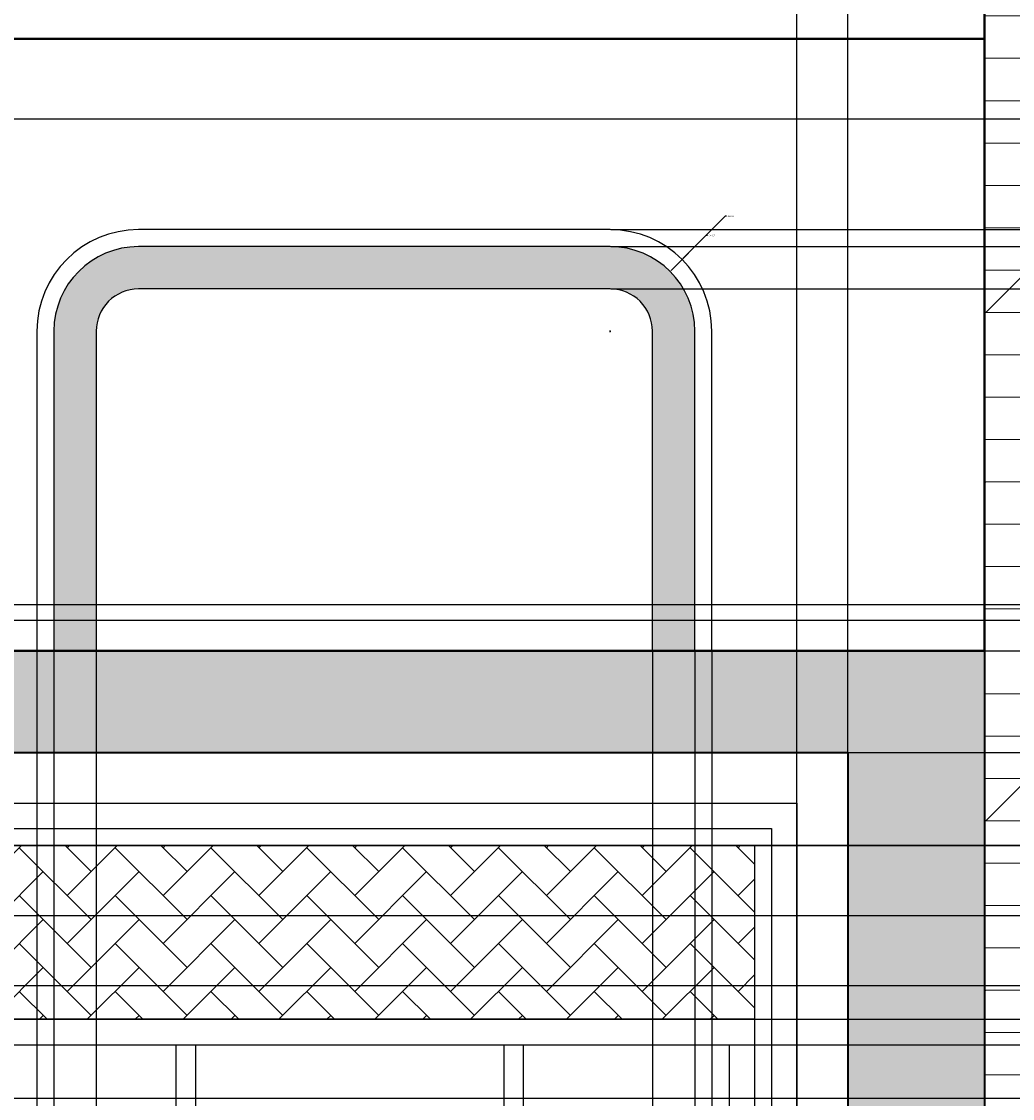
# Model space of a CAD drawing. Units: inches. Extents: x -13 to 630, y -103 to 275.
# Tile 4 of 9: x 51 to 168, y 72 to 199. Entities that reach past the tile are written whole.
import ezdxf

# ---------------------------------------------------------------- set-up
doc = ezdxf.new("R2010")
doc.units = ezdxf.units.IN
doc.header["$MEASUREMENT"] = 0
for name, color, linetype, lineweight in [('A-ANNO-DIMS', 2, 'Continuous', 18), ('A-ELEV', 7, 'Continuous', 35), ('A-ELEV-PATT', 8, 'Continuous', 13), ('A-GLAZ', 4, 'Continuous', 25)]:
    doc.layers.add(name, color=color, linetype=linetype, lineweight=lineweight)
doc.styles.get("Standard").update_dxf_attribs({"font": 'arial.ttf'})
doc.dimstyles.get("Standard").update_dxf_attribs({"dimtxt": 0.18, "dimasz": 0.18, "dimexe": 0.18, "dimexo": 0.0625, "dimgap": 0.09, "dimtad": 0, "dimtih": 1, "dimtoh": 1, "dimdec": 4, "dimzin": 0, "dimdsep": 46, "dimtxsty": 'Standard', "dimcen": 0.09, "dimadec": 0, "dimazin": 0, "dimtfac": 1, "dimtdec": 4, "dimtofl": 0, "dimtmove": 0, "dimatfit": 3, "dimfxl": 1, "dimtolj": 1, "dimtzin": 0, "dimarcsym": 0})

# ---------------------------------------------------------------- blocks, each defined once
blk = doc.blocks.new('WIN-GROUND')
for points in [[(0, 0), (0, 102), (108, 102), (108, 0)], [(3, 0), (3, 99), (105, 99), (105, 0)], [(5, 0), (5, 97), (103, 97), (103, 0)], [(34.74, 56.82), (34.74, 73.49), (37, 73.49), (37, 56.82)], [(73.43, 56.82), (73.43, 73.49), (75.7, 73.49), (75.7, 56.82)], [(34.74, 55.51), (8, 55.51), (8, 56.82), (34.74, 56.82)], [(37, 56.82), (73.43, 56.82)], [(75.7, 56.82), (100, 56.82), (100, 55.51), (75.7, 55.51)], [(34.74, 21.58), (34.74, 55.51)], [(37, 55.51), (37, 21.58)], [(73.43, 55.51), (37, 55.51)], [(73.43, 21.58), (73.43, 55.51)], [(75.7, 55.51), (75.7, 21.58)], [(34.74, 20.27), (8, 20.27), (8, 21.58), (34.74, 21.58)], [(37, 21.58), (73.43, 21.58)], [(75.7, 21.58), (100, 21.58), (100, 20.27), (75.7, 20.27)], [(37, 20.27), (37, 3), (34.74, 3), (34.74, 20.27)], [(73.43, 20.27), (37, 20.27)], [(75.7, 20.27), (75.7, 3), (73.43, 3), (73.43, 20.27)]]:
    blk.add_lwpolyline(points)
for points in [[(5, 97), (103, 97), (103, 76.49), (5, 76.49)], [(5, 76.49), (103, 76.49), (103, 0), (5, 0)], [(8, 73.49), (100, 73.49), (100, 3), (8, 3)]]:
    blk.add_lwpolyline(points, close=True)
blk = doc.blocks.new('*D8')
at = {"layer": 'A-ANNO-DIMS', "color": 0, "lineweight": -2, "transparency": 16777216}
for p, q in [((142.71, 5.14), (142.71, 275.01)), ((142.89, 274.83), (153.31, 274.83)), ((164.66, 274.83), (154.24, 274.83)), ((164.84, 5.14), (164.84, 275.01))]:
    blk.add_line(p, q, dxfattribs=at)
at = {"layer": 'A-ANNO-DIMS', "color": 0, "transparency": 16777216}
for points in [[(142.89, 274.86), (142.89, 274.8), (142.71, 274.83)], [(164.66, 274.86), (164.66, 274.8), (164.84, 274.83)]]:
    blk.add_solid(points, dxfattribs=at)
at = {"layer": 'Defpoints', "color": 0, "transparency": 16777216}
for p in [(164.84, 274.83), (142.71, 5.08), (164.84, 5.08)]:
    blk.add_point(p, dxfattribs=at)
at = {"layer": 'A-ANNO-DIMS', "color": 0, "transparency": 16777216, "insert": (153.78, 274.83), "char_height": 0.18, "attachment_point": 5}
blk.add_mtext('\\A1;22.133', dxfattribs=at)
blk = doc.blocks.new('*D41')
at = {"layer": 'A-ANNO-DIMS', "color": 0, "lineweight": -2, "transparency": 16777216}
for p, q in [((205.96, 72.22), (-13.22, 72.22)), ((-13.04, 72.04), (-13.04, 71.07)), ((-13.04, 69.73), (-13.04, 70.7)), ((205.96, 69.55), (-13.22, 69.55))]:
    blk.add_line(p, q, dxfattribs=at)
at = {"layer": 'A-ANNO-DIMS', "color": 0, "transparency": 16777216}
for points in [[(-13.07, 72.04), (-13.01, 72.04), (-13.04, 72.22)], [(-13.07, 69.73), (-13.01, 69.73), (-13.04, 69.55)]]:
    blk.add_solid(points, dxfattribs=at)
at = {"layer": 'Defpoints', "color": 0, "transparency": 16777216}
for p in [(-13.04, 72.22), (206.02, 72.22), (206.02, 69.55)]:
    blk.add_point(p, dxfattribs=at)
at = {"layer": 'A-ANNO-DIMS', "color": 0, "transparency": 16777216, "insert": (-13.04, 70.88), "char_height": 0.18, "attachment_point": 5}
blk.add_mtext('\\A1;2.68', dxfattribs=at)
blk = doc.blocks.new('*D42')
at = {"layer": 'A-ANNO-DIMS', "color": 0, "lineweight": -2, "transparency": 16777216}
for p, q in [((205.96, 85.52), (-13.22, 85.52)), ((-13.04, 85.34), (-13.04, 79.05)), ((-13.04, 72.4), (-13.04, 78.69)), ((205.96, 72.22), (-13.22, 72.22))]:
    blk.add_line(p, q, dxfattribs=at)
at = {"layer": 'A-ANNO-DIMS', "color": 0, "transparency": 16777216}
for points in [[(-13.07, 85.34), (-13.01, 85.34), (-13.04, 85.52)], [(-13.07, 72.4), (-13.01, 72.4), (-13.04, 72.22)]]:
    blk.add_solid(points, dxfattribs=at)
at = {"layer": 'Defpoints', "color": 0, "transparency": 16777216}
for p in [(-13.04, 85.52), (206.02, 85.52), (206.02, 72.22)]:
    blk.add_point(p, dxfattribs=at)
at = {"layer": 'A-ANNO-DIMS', "color": 0, "transparency": 16777216, "insert": (-13.04, 78.87), "char_height": 0.18, "attachment_point": 5}
blk.add_mtext('\\A1;13.297', dxfattribs=at)
blk = doc.blocks.new('*D43')
at = {"layer": 'A-ANNO-DIMS', "color": 0, "lineweight": -2, "transparency": 16777216}
for p, q in [((205.96, 93.8), (-13.22, 93.8)), ((-13.04, 93.62), (-13.04, 89.84)), ((-13.04, 85.7), (-13.04, 89.48)), ((205.96, 85.52), (-13.22, 85.52))]:
    blk.add_line(p, q, dxfattribs=at)
at = {"layer": 'A-ANNO-DIMS', "color": 0, "transparency": 16777216}
for points in [[(-13.07, 93.62), (-13.01, 93.62), (-13.04, 93.8)], [(-13.07, 85.7), (-13.01, 85.7), (-13.04, 85.52)]]:
    blk.add_solid(points, dxfattribs=at)
at = {"layer": 'Defpoints', "color": 0, "transparency": 16777216}
for p in [(-13.04, 93.8), (206.02, 93.8), (206.02, 85.52)]:
    blk.add_point(p, dxfattribs=at)
at = {"layer": 'A-ANNO-DIMS', "color": 0, "transparency": 16777216, "insert": (-13.04, 89.66), "char_height": 0.18, "attachment_point": 5}
blk.add_mtext('\\A1;8.28', dxfattribs=at)
blk = doc.blocks.new('*D44')
at = {"layer": 'A-ANNO-DIMS', "color": 0, "lineweight": -2, "transparency": 16777216}
for p, q in [((205.96, 102.08), (-13.22, 102.08)), ((-13.04, 101.9), (-13.04, 98.12)), ((-13.04, 93.98), (-13.04, 97.76)), ((205.96, 93.8), (-13.22, 93.8))]:
    blk.add_line(p, q, dxfattribs=at)
at = {"layer": 'A-ANNO-DIMS', "color": 0, "transparency": 16777216}
for points in [[(-13.07, 101.9), (-13.01, 101.9), (-13.04, 102.08)], [(-13.07, 93.98), (-13.01, 93.98), (-13.04, 93.8)]]:
    blk.add_solid(points, dxfattribs=at)
at = {"layer": 'Defpoints', "color": 0, "transparency": 16777216}
for p in [(-13.04, 102.08), (206.02, 102.08), (206.02, 93.8)]:
    blk.add_point(p, dxfattribs=at)
at = {"layer": 'A-ANNO-DIMS', "color": 0, "transparency": 16777216, "insert": (-13.04, 97.94), "char_height": 0.18, "attachment_point": 5}
blk.add_mtext('\\A1;8.28', dxfattribs=at)
blk = doc.blocks.new('*D45')
at = {"layer": 'A-ANNO-DIMS', "color": 0, "lineweight": -2, "transparency": 16777216}
for p, q in [((205.96, 128.66), (-13.22, 128.66)), ((-13.04, 128.48), (-13.04, 115.55)), ((-13.04, 102.26), (-13.04, 115.19)), ((205.96, 102.08), (-13.22, 102.08))]:
    blk.add_line(p, q, dxfattribs=at)
at = {"layer": 'A-ANNO-DIMS', "color": 0, "transparency": 16777216}
for points in [[(-13.07, 128.48), (-13.01, 128.48), (-13.04, 128.66)], [(-13.07, 102.26), (-13.01, 102.26), (-13.04, 102.08)]]:
    blk.add_solid(points, dxfattribs=at)
at = {"layer": 'Defpoints', "color": 0, "transparency": 16777216}
for p in [(-13.04, 128.66), (206.02, 128.66), (206.02, 102.08)]:
    blk.add_point(p, dxfattribs=at)
at = {"layer": 'A-ANNO-DIMS', "color": 0, "transparency": 16777216, "insert": (-13.04, 115.37), "char_height": 0.18, "attachment_point": 5}
blk.add_mtext('\\A1;26.574', dxfattribs=at)
blk = doc.blocks.new('*D46')
at = {"layer": 'A-ANNO-DIMS', "color": 0, "lineweight": -2, "transparency": 16777216}
for p, q in [((205.96, 130.51), (-13.22, 130.51)), ((-13.04, 130.33), (-13.04, 129.76)), ((205.96, 128.66), (-13.22, 128.66)), ((-13.04, 128.84), (-13.04, 129.4))]:
    blk.add_line(p, q, dxfattribs=at)
at = {"layer": 'A-ANNO-DIMS', "color": 0, "transparency": 16777216}
for points in [[(-13.07, 130.33), (-13.01, 130.33), (-13.04, 130.51)], [(-13.07, 128.84), (-13.01, 128.84), (-13.04, 128.66)]]:
    blk.add_solid(points, dxfattribs=at)
at = {"layer": 'Defpoints', "color": 0, "transparency": 16777216}
for p in [(-13.04, 130.51), (206.02, 130.51), (206.02, 128.66)]:
    blk.add_point(p, dxfattribs=at)
at = {"layer": 'A-ANNO-DIMS', "color": 0, "transparency": 16777216, "insert": (-13.04, 129.58), "char_height": 0.18, "attachment_point": 5}
blk.add_mtext('\\A1;1.854', dxfattribs=at)
blk = doc.blocks.new('*D47')
at = {"layer": 'A-ANNO-DIMS', "color": 0, "lineweight": -2, "transparency": 16777216}
for p, q in [((252.21, 187.83), (-13.22, 187.83)), ((-13.04, 187.65), (-13.04, 159.35)), ((-13.04, 130.69), (-13.04, 158.99)), ((205.96, 130.51), (-13.22, 130.51))]:
    blk.add_line(p, q, dxfattribs=at)
at = {"layer": 'A-ANNO-DIMS', "color": 0, "transparency": 16777216}
for points in [[(-13.07, 187.65), (-13.01, 187.65), (-13.04, 187.83)], [(-13.07, 130.69), (-13.01, 130.69), (-13.04, 130.51)]]:
    blk.add_solid(points, dxfattribs=at)
at = {"layer": 'Defpoints', "color": 0, "transparency": 16777216}
for p in [(-13.04, 187.83), (252.27, 187.83), (206.02, 130.51)]:
    blk.add_point(p, dxfattribs=at)
at = {"layer": 'A-ANNO-DIMS', "color": 0, "transparency": 16777216, "insert": (-13.04, 159.17), "char_height": 0.18, "attachment_point": 5}
blk.add_mtext('\\A1;57.32', dxfattribs=at)
blk = doc.blocks.new('*D70')
at = {"layer": 'A-ANNO-DIMS', "color": 0, "lineweight": -2, "transparency": 16777216}
for p, q in [((142.71, 107.14), (142.71, 275.01)), ((142.89, 274.83), (145.56, 274.83)), ((148.53, 274.83), (145.86, 274.83)), ((148.71, 113.14), (148.71, 275.01))]:
    blk.add_line(p, q, dxfattribs=at)
at = {"layer": 'A-ANNO-DIMS', "color": 0, "transparency": 16777216}
for points in [[(142.89, 274.86), (142.89, 274.8), (142.71, 274.83)], [(148.53, 274.86), (148.53, 274.8), (148.71, 274.83)]]:
    blk.add_solid(points, dxfattribs=at)
at = {"layer": 'Defpoints', "color": 0, "transparency": 16777216}
for p in [(148.71, 274.83), (148.71, 113.08), (142.71, 107.08)]:
    blk.add_point(p, dxfattribs=at)
at = {"layer": 'A-ANNO-DIMS', "color": 0, "transparency": 16777216, "insert": (145.71, 274.83), "char_height": 0.18, "attachment_point": 5}
blk.add_mtext('\\A1;6', dxfattribs=at)
blk = doc.blocks.new('*D83')
at = {"layer": 'A-ANNO-DIMS', "color": 0, "lineweight": -2, "transparency": 16777216}
for p, q in [((134.77, 78.57), (630.03, 78.57)), ((629.85, 78.39), (629.85, 70.42)), ((629.85, 62.08), (629.85, 70.05)), ((134.77, 61.9), (630.03, 61.9))]:
    blk.add_line(p, q, dxfattribs=at)
at = {"layer": 'A-ANNO-DIMS', "color": 0, "transparency": 16777216}
for points in [[(629.82, 78.39), (629.88, 78.39), (629.85, 78.57)], [(629.82, 62.08), (629.88, 62.08), (629.85, 61.9)]]:
    blk.add_solid(points, dxfattribs=at)
at = {"layer": 'Defpoints', "color": 0, "transparency": 16777216}
for p in [(134.71, 78.57), (629.85, 78.57), (134.71, 61.9)]:
    blk.add_point(p, dxfattribs=at)
at = {"layer": 'A-ANNO-DIMS', "color": 0, "transparency": 16777216, "insert": (629.85, 70.24), "char_height": 0.18, "attachment_point": 5}
blk.add_mtext('\\A1;16.67', dxfattribs=at)
blk = doc.blocks.new('*D84')
at = {"layer": 'A-ANNO-DIMS', "color": 0, "lineweight": -2, "transparency": 16777216}
for p, q in [((137.77, 81.57), (630.03, 81.57)), ((629.85, 81.39), (629.85, 80.25)), ((629.85, 78.75), (629.85, 79.89)), ((134.77, 78.57), (630.03, 78.57))]:
    blk.add_line(p, q, dxfattribs=at)
at = {"layer": 'A-ANNO-DIMS', "color": 0, "transparency": 16777216}
for points in [[(629.82, 81.39), (629.88, 81.39), (629.85, 81.57)], [(629.82, 78.75), (629.88, 78.75), (629.85, 78.57)]]:
    blk.add_solid(points, dxfattribs=at)
at = {"layer": 'Defpoints', "color": 0, "transparency": 16777216}
for p in [(137.71, 81.57), (629.85, 81.57), (134.71, 78.57)]:
    blk.add_point(p, dxfattribs=at)
at = {"layer": 'A-ANNO-DIMS', "color": 0, "transparency": 16777216, "insert": (629.85, 80.07), "char_height": 0.18, "attachment_point": 5}
blk.add_mtext('\\A1;3', dxfattribs=at)
blk = doc.blocks.new('*D85')
at = {"layer": 'A-ANNO-DIMS', "color": 0, "lineweight": -2, "transparency": 16777216}
for p, q in [((137.77, 102.08), (630.03, 102.08)), ((629.85, 101.9), (629.85, 92.01)), ((629.85, 81.75), (629.85, 91.64)), ((137.77, 81.57), (630.03, 81.57))]:
    blk.add_line(p, q, dxfattribs=at)
at = {"layer": 'A-ANNO-DIMS', "color": 0, "transparency": 16777216}
for points in [[(629.82, 101.9), (629.88, 101.9), (629.85, 102.08)], [(629.82, 81.75), (629.88, 81.75), (629.85, 81.57)]]:
    blk.add_solid(points, dxfattribs=at)
at = {"layer": 'Defpoints', "color": 0, "transparency": 16777216}
for p in [(137.71, 102.08), (629.85, 102.08), (137.71, 81.57)]:
    blk.add_point(p, dxfattribs=at)
at = {"layer": 'A-ANNO-DIMS', "color": 0, "transparency": 16777216, "insert": (629.85, 91.83), "char_height": 0.18, "attachment_point": 5}
blk.add_mtext('\\A1;20.51', dxfattribs=at)
blk = doc.blocks.new('*D86')
at = {"layer": 'A-ANNO-DIMS', "color": 0, "lineweight": -2, "transparency": 16777216}
for p, q in [((148.77, 113.08), (630.03, 113.08)), ((629.85, 112.9), (629.85, 107.76)), ((629.85, 102.26), (629.85, 107.4)), ((137.77, 102.08), (630.03, 102.08))]:
    blk.add_line(p, q, dxfattribs=at)
at = {"layer": 'A-ANNO-DIMS', "color": 0, "transparency": 16777216}
for points in [[(629.82, 112.9), (629.88, 112.9), (629.85, 113.08)], [(629.82, 102.26), (629.88, 102.26), (629.85, 102.08)]]:
    blk.add_solid(points, dxfattribs=at)
at = {"layer": 'Defpoints', "color": 0, "transparency": 16777216}
for p in [(148.71, 113.08), (629.85, 113.08), (137.71, 102.08)]:
    blk.add_point(p, dxfattribs=at)
at = {"layer": 'A-ANNO-DIMS', "color": 0, "transparency": 16777216, "insert": (629.85, 107.58), "char_height": 0.18, "attachment_point": 5}
blk.add_mtext('\\A1;11', dxfattribs=at)
blk = doc.blocks.new('*D106')
at = {"layer": 'A-ANNO-DIMS', "color": 0, "lineweight": -2, "transparency": 16777216}
for p, q in [((42.29, 125.02), (42.29, -103.45)), ((53, 125.02), (53, -103.45)), ((42.47, -103.27), (47.27, -103.27)), ((52.82, -103.27), (48.01, -103.27))]:
    blk.add_line(p, q, dxfattribs=at)
at = {"layer": 'A-ANNO-DIMS', "color": 0, "transparency": 16777216}
for points in [[(42.47, -103.24), (42.47, -103.3), (42.29, -103.27)], [(52.82, -103.24), (52.82, -103.3), (53, -103.27)]]:
    blk.add_solid(points, dxfattribs=at)
at = {"layer": 'Defpoints', "color": 0, "transparency": 16777216}
for p in [(42.29, 125.08), (53, 125.08), (53, -103.27)]:
    blk.add_point(p, dxfattribs=at)
at = {"layer": 'A-ANNO-DIMS', "color": 0, "transparency": 16777216, "insert": (47.64, -103.27), "char_height": 0.18, "attachment_point": 5}
blk.add_mtext('\\A1;10.71', dxfattribs=at)
blk = doc.blocks.new('*D107')
at = {"layer": 'A-ANNO-DIMS', "color": 0, "lineweight": -2, "transparency": 16777216}
for p, q in [((53, 125.02), (53, -103.45)), ((55, 125.02), (55, -103.45)), ((53.18, -103.27), (53.85, -103.27)), ((54.82, -103.27), (54.14, -103.27))]:
    blk.add_line(p, q, dxfattribs=at)
at = {"layer": 'A-ANNO-DIMS', "color": 0, "transparency": 16777216}
for points in [[(53.18, -103.24), (53.18, -103.3), (53, -103.27)], [(54.82, -103.24), (54.82, -103.3), (55, -103.27)]]:
    blk.add_solid(points, dxfattribs=at)
at = {"layer": 'Defpoints', "color": 0, "transparency": 16777216}
for p in [(53, 125.08), (55, 125.08), (55, -103.27)]:
    blk.add_point(p, dxfattribs=at)
at = {"layer": 'A-ANNO-DIMS', "color": 0, "transparency": 16777216, "insert": (54, -103.27), "char_height": 0.18, "attachment_point": 5}
blk.add_mtext('\\A1;2', dxfattribs=at)
blk = doc.blocks.new('*D108')
at = {"layer": 'A-ANNO-DIMS', "color": 0, "lineweight": -2, "transparency": 16777216}
for p, q in [((55, 125.02), (55, -103.45)), ((60, 125.02), (60, -103.45)), ((55.18, -103.27), (57.35, -103.27)), ((59.82, -103.27), (57.64, -103.27))]:
    blk.add_line(p, q, dxfattribs=at)
at = {"layer": 'A-ANNO-DIMS', "color": 0, "transparency": 16777216}
for points in [[(55.18, -103.24), (55.18, -103.3), (55, -103.27)], [(59.82, -103.24), (59.82, -103.3), (60, -103.27)]]:
    blk.add_solid(points, dxfattribs=at)
at = {"layer": 'Defpoints', "color": 0, "transparency": 16777216}
for p in [(55, 125.08), (60, 125.08), (60, -103.27)]:
    blk.add_point(p, dxfattribs=at)
at = {"layer": 'A-ANNO-DIMS', "color": 0, "transparency": 16777216, "insert": (57.5, -103.27), "char_height": 0.18, "attachment_point": 5}
blk.add_mtext('\\A1;5', dxfattribs=at)
blk = doc.blocks.new('*D109')
at = {"layer": 'A-ANNO-DIMS', "color": 0, "lineweight": -2, "transparency": 16777216}
for p, q in [((60, 125.02), (60, -103.45)), ((125.66, 125.02), (125.66, -103.45)), ((60.18, -103.27), (92.44, -103.27)), ((125.48, -103.27), (93.22, -103.27))]:
    blk.add_line(p, q, dxfattribs=at)
at = {"layer": 'A-ANNO-DIMS', "color": 0, "transparency": 16777216}
for points in [[(60.18, -103.24), (60.18, -103.3), (60, -103.27)], [(125.48, -103.24), (125.48, -103.3), (125.66, -103.27)]]:
    blk.add_solid(points, dxfattribs=at)
at = {"layer": 'Defpoints', "color": 0, "transparency": 16777216}
for p in [(60, 125.08), (125.66, 125.08), (125.66, -103.27)]:
    blk.add_point(p, dxfattribs=at)
at = {"layer": 'A-ANNO-DIMS', "color": 0, "transparency": 16777216, "insert": (92.83, -103.27), "char_height": 0.18, "attachment_point": 5}
blk.add_mtext('\\A1;65.67', dxfattribs=at)
blk = doc.blocks.new('*D110')
at = {"layer": 'A-ANNO-DIMS', "color": 0, "lineweight": -2, "transparency": 16777216}
for p, q in [((125.66, 125.02), (125.66, -103.45)), ((130.66, 125.02), (130.66, -103.45)), ((125.84, -103.27), (128.01, -103.27)), ((130.48, -103.27), (128.31, -103.27))]:
    blk.add_line(p, q, dxfattribs=at)
at = {"layer": 'A-ANNO-DIMS', "color": 0, "transparency": 16777216}
for points in [[(125.84, -103.24), (125.84, -103.3), (125.66, -103.27)], [(130.48, -103.24), (130.48, -103.3), (130.66, -103.27)]]:
    blk.add_solid(points, dxfattribs=at)
at = {"layer": 'Defpoints', "color": 0, "transparency": 16777216}
for p in [(125.66, 125.08), (130.66, 125.08), (130.66, -103.27)]:
    blk.add_point(p, dxfattribs=at)
at = {"layer": 'A-ANNO-DIMS', "color": 0, "transparency": 16777216, "insert": (128.16, -103.27), "char_height": 0.18, "attachment_point": 5}
blk.add_mtext('\\A1;5', dxfattribs=at)
blk = doc.blocks.new('*D111')
at = {"layer": 'A-ANNO-DIMS', "color": 0, "lineweight": -2, "transparency": 16777216}
for p, q in [((130.66, 125.02), (130.66, -103.45)), ((132.66, 125.02), (132.66, -103.45)), ((130.84, -103.27), (131.51, -103.27)), ((132.48, -103.27), (131.81, -103.27))]:
    blk.add_line(p, q, dxfattribs=at)
at = {"layer": 'A-ANNO-DIMS', "color": 0, "transparency": 16777216}
for points in [[(130.84, -103.24), (130.84, -103.3), (130.66, -103.27)], [(132.48, -103.24), (132.48, -103.3), (132.66, -103.27)]]:
    blk.add_solid(points, dxfattribs=at)
at = {"layer": 'Defpoints', "color": 0, "transparency": 16777216}
for p in [(130.66, 125.08), (132.66, 125.08), (132.66, -103.27)]:
    blk.add_point(p, dxfattribs=at)
at = {"layer": 'A-ANNO-DIMS', "color": 0, "transparency": 16777216, "insert": (131.66, -103.27), "char_height": 0.18, "attachment_point": 5}
blk.add_mtext('\\A1;2', dxfattribs=at)
blk = doc.blocks.new('*D112')
at = {"layer": 'A-ANNO-DIMS', "color": 0, "lineweight": -2, "transparency": 16777216}
for p, q in [((132.66, 125.02), (132.66, -103.45)), ((164.84, 125.02), (164.84, -103.45)), ((132.84, -103.27), (148.36, -103.27)), ((164.66, -103.27), (149.15, -103.27))]:
    blk.add_line(p, q, dxfattribs=at)
at = {"layer": 'A-ANNO-DIMS', "color": 0, "transparency": 16777216}
for points in [[(132.84, -103.24), (132.84, -103.3), (132.66, -103.27)], [(164.66, -103.24), (164.66, -103.3), (164.84, -103.27)]]:
    blk.add_solid(points, dxfattribs=at)
at = {"layer": 'Defpoints', "color": 0, "transparency": 16777216}
for p in [(132.66, 125.08), (164.84, 125.08), (164.84, -103.27)]:
    blk.add_point(p, dxfattribs=at)
at = {"layer": 'A-ANNO-DIMS', "color": 0, "transparency": 16777216, "insert": (148.75, -103.27), "char_height": 0.18, "attachment_point": 5}
blk.add_mtext('\\A1;32.18', dxfattribs=at)
blk = doc.blocks.new('*D113')
at = {"layer": 'A-ANNO-DIMS', "color": 0, "lineweight": -2, "transparency": 16777216}
for p, q in [((120.73, 167.79), (630.03, 167.79)), ((629.85, 167.61), (629.85, 146.61)), ((629.85, 125.26), (629.85, 146.25)), ((132.73, 125.08), (630.03, 125.08))]:
    blk.add_line(p, q, dxfattribs=at)
at = {"layer": 'A-ANNO-DIMS', "color": 0, "transparency": 16777216}
for points in [[(629.82, 167.61), (629.88, 167.61), (629.85, 167.79)], [(629.82, 125.26), (629.88, 125.26), (629.85, 125.08)]]:
    blk.add_solid(points, dxfattribs=at)
at = {"layer": 'Defpoints', "color": 0, "transparency": 16777216}
for p in [(120.66, 167.79), (629.85, 167.79), (132.66, 125.08)]:
    blk.add_point(p, dxfattribs=at)
at = {"layer": 'A-ANNO-DIMS', "color": 0, "transparency": 16777216, "insert": (629.85, 146.43), "char_height": 0.18, "attachment_point": 5}
blk.add_mtext('\\A1;42.705', dxfattribs=at)
blk = doc.blocks.new('*D114')
at = {"layer": 'A-ANNO-DIMS', "color": 0, "lineweight": -2, "transparency": 16777216}
for p, q in [((120.73, 172.79), (630.03, 172.79)), ((629.85, 172.61), (629.85, 170.47)), ((629.85, 167.97), (629.85, 170.1)), ((120.73, 167.79), (630.03, 167.79))]:
    blk.add_line(p, q, dxfattribs=at)
at = {"layer": 'A-ANNO-DIMS', "color": 0, "transparency": 16777216}
for points in [[(629.82, 172.61), (629.88, 172.61), (629.85, 172.79)], [(629.82, 167.97), (629.88, 167.97), (629.85, 167.79)]]:
    blk.add_solid(points, dxfattribs=at)
at = {"layer": 'Defpoints', "color": 0, "transparency": 16777216}
for p in [(120.66, 172.79), (629.85, 172.79), (120.66, 167.79)]:
    blk.add_point(p, dxfattribs=at)
at = {"layer": 'A-ANNO-DIMS', "color": 0, "transparency": 16777216, "insert": (629.85, 170.29), "char_height": 0.18, "attachment_point": 5}
blk.add_mtext('\\A1;5', dxfattribs=at)
blk = doc.blocks.new('*D115')
at = {"layer": 'A-ANNO-DIMS', "color": 0, "lineweight": -2, "transparency": 16777216}
for p, q in [((120.73, 174.79), (630.03, 174.79)), ((629.85, 174.61), (629.85, 173.97)), ((629.85, 172.97), (629.85, 173.6)), ((120.73, 172.79), (630.03, 172.79))]:
    blk.add_line(p, q, dxfattribs=at)
at = {"layer": 'A-ANNO-DIMS', "color": 0, "transparency": 16777216}
for points in [[(629.82, 174.61), (629.88, 174.61), (629.85, 174.79)], [(629.82, 172.97), (629.88, 172.97), (629.85, 172.79)]]:
    blk.add_solid(points, dxfattribs=at)
at = {"layer": 'Defpoints', "color": 0, "transparency": 16777216}
for p in [(120.66, 174.79), (629.85, 174.79), (120.66, 172.79)]:
    blk.add_point(p, dxfattribs=at)
at = {"layer": 'A-ANNO-DIMS', "color": 0, "transparency": 16777216, "insert": (629.85, 173.79), "char_height": 0.18, "attachment_point": 5}
blk.add_mtext('\\A1;2', dxfattribs=at)
blk = doc.blocks.new('*D122')
at = {"layer": 'A-ANNO-DIMS', "color": 0, "lineweight": -2, "transparency": 16777216}
for p, q in [((134.24, 176.36), (129.28, 171.4)), ((134.42, 176.36), (134.24, 176.36)), ((120.57, 162.79), (120.75, 162.79)), ((120.66, 162.7), (120.66, 162.88))]:
    blk.add_line(p, q, dxfattribs=at)
at = {"layer": 'A-ANNO-DIMS', "color": 0, "transparency": 16777216}
blk.add_solid([(129.26, 171.42), (129.3, 171.38), (129.15, 171.27)], dxfattribs=at)
at = {"layer": 'Defpoints', "color": 0, "transparency": 16777216}
for p in [(129.15, 171.27), (120.66, 162.79)]:
    blk.add_point(p, dxfattribs=at)
at = {"layer": 'A-ANNO-DIMS', "color": 0, "transparency": 16777216, "insert": (134.92, 176.36), "char_height": 0.18, "attachment_point": 5}
blk.add_mtext('\\A1;4X R12', dxfattribs=at)
blk = doc.blocks.new('*D123')
at = {"layer": 'A-ANNO-DIMS', "color": 0, "lineweight": -2, "transparency": 16777216}
for p, q in [((131.98, 174.1), (127.86, 169.98)), ((132.16, 174.1), (131.98, 174.1)), ((120.57, 162.79), (120.75, 162.79)), ((120.66, 162.7), (120.66, 162.88))]:
    blk.add_line(p, q, dxfattribs=at)
at = {"layer": 'A-ANNO-DIMS', "color": 0, "transparency": 16777216}
blk.add_solid([(127.84, 170), (127.88, 169.96), (127.74, 169.86)], dxfattribs=at)
at = {"layer": 'Defpoints', "color": 0, "transparency": 16777216}
for p in [(127.74, 169.86), (120.66, 162.79)]:
    blk.add_point(p, dxfattribs=at)
at = {"layer": 'A-ANNO-DIMS', "color": 0, "transparency": 16777216, "insert": (132.66, 174.1), "char_height": 0.18, "attachment_point": 5}
blk.add_mtext('\\A1;4X R10', dxfattribs=at)

msp = doc.modelspace()

# ---------------------------------------------------------------- hatches: boundary and pattern name
at = {"layer": 'A-ELEV-PATT', "transparency": 33554541}
h = msp.add_hatch(dxfattribs=at)
h.set_pattern_fill('DOLMIT', color=256, scale=20)
h.paths.add_polyline_path([(345.3061, 245.0808), (164.8443, 245.0808), (164.8443, 5.0808), (176.8443, 5.0808), (176.8443, 233.0808), (333.3061, 233.0808), (333.3061, 5.0808), (345.3061, 5.0808)])
at = {"layer": 'A-ELEV-PATT'}
h = msp.add_hatch(dxfattribs=at)
h.set_pattern_fill('BRSTONE', color=256, scale=20)
h.paths.add_polyline_path([(120.6641, 172.7854), (64.9953, 172.7854, 0.41421356), (54.9953, 162.7854), (54.9953, 125.0808), (59.9953, 125.0808), (59.9953, 162.7854, -0.41421356), (64.9953, 167.7854), (120.6641, 167.7854, -0.41421356), (125.6641, 162.7854), (125.6641, 125.0808), (130.6641, 125.0808), (130.6641, 162.7854, 0.41421356)])
h.paths.add_polyline_path([(439.5513, 172.7854), (383.8825, 172.7854, 0.41421356), (373.8825, 162.7854), (373.8825, 125.0808), (378.8825, 125.0808), (378.8825, 162.7854, -0.41421356), (383.8825, 167.7854), (439.5513, 167.7854, -0.41421356), (444.5513, 162.7854), (444.5513, 125.0808), (449.5513, 125.0808), (449.5513, 162.7854, 0.41421356)])
h.paths.add_polyline_path([(364.7117, 113.0808), (484.7117, 113.0808), (484.7117, 5.0808), (496.7117, 5.0808), (496.7117, 125.0808), (345.3061, 125.0808), (345.3061, 5.0808), (364.7117, 5.0808)])
h.paths.add_polyline_path([(164.8443, 125.0808), (28.7117, 125.0808), (16.7117, 125.0808), (16.7117, 5.0808), (28.7117, 5.0808), (28.7117, 113.0808), (148.7117, 113.0808), (148.7117, 5.0808), (164.8443, 5.0808)])
h.paths.add_polyline_path([(95.1171, 223.9392), (83.8622, 223.9392), (83.8622, 206.5279), (95.1171, 206.5279)])
h.paths.add_polyline_path([(54.9212, 223.9392), (40.7186, 223.9392), (40.7186, 206.5279), (54.9212, 206.5279)])
h.paths.add_polyline_path([(463.828, 223.9392), (449.6254, 223.9392), (449.6254, 206.5279), (463.828, 206.5279)])
h.paths.add_polyline_path([(420.6843, 223.9392), (409.4295, 223.9392), (409.4295, 206.5279), (420.6843, 206.5279)])
h = msp.add_hatch(dxfattribs=at)
h.set_pattern_fill('STEEL', color=256, scale=20)
h.set_pattern_definition([(45, (0, 0), (-1.767767, 1.767767), []), (45, (0, 1.25), (-1.767767, 1.767767), [])])
h.paths.add_polyline_path([(164.8443, 218.2056), (95.1171, 218.2056), (95.1171, 215.2335), (164.8443, 215.2335)])
h.paths.add_polyline_path([(83.8622, 218.2056), (54.9212, 218.2056), (54.9212, 215.2335), (83.8622, 215.2335)])
h.paths.add_polyline_path([(409.4295, 218.2056), (345.3061, 218.2056), (345.3061, 215.2335), (409.4295, 215.2335)])
h.paths.add_polyline_path([(449.6254, 218.2056), (420.6843, 218.2056), (420.6843, 215.2335), (449.6254, 215.2335)])
h.paths.add_polyline_path([(302.5258, 203.9359), (202.0208, 203.9359), (202.0208, 128.6551, -0.36718729), (252.2733, 187.858, -0.36718729), (302.5258, 128.6551)])
h = msp.add_hatch(dxfattribs=at)
h.set_pattern_fill('AR-HBONE', color=256)
h.paths.add_polyline_path([(137.7117, 102.0808), (39.7117, 102.0808), (39.7117, 81.5713), (137.7117, 81.5713)])
h.paths.add_polyline_path([(473.7117, 102.0808), (375.7117, 102.0808), (375.7117, 81.5713), (473.7117, 81.5713)])

# ---------------------------------------------------------------- linework, layer by layer
at = {"layer": 'A-ELEV'}
msp.add_line((52.9953, 125.0808), (132.6641, 125.0808), dxfattribs=at)
for points in [[(345.3061, 5.0808), (345.3061, 245.0808), (164.8443, 245.0808), (164.8443, 5.0808)], [(164.8443, 125.0808), (16.7117, 125.0808), (16.7117, 5.0808)], [(28.7117, 5.0808), (28.7117, 113.0808), (148.7117, 113.0808), (148.7117, 5.0808)]]:
    msp.add_lwpolyline(points, dxfattribs=at)
for points in [[(18.8732, 197.3216), (164.8443, 197.3216), (164.8443, 206.5279), (18.8732, 206.5279)], [(28.7117, 125.0808), (164.8443, 125.0808), (164.8443, 197.3216), (28.7117, 197.3216)]]:
    msp.add_lwpolyline(points, close=True, dxfattribs=at)
at = {"layer": 'A-GLAZ'}
for points in [[(132.6641, 125.0808), (132.6641, 162.7854, 0.41421356), (120.6641, 174.7854), (64.9953, 174.7854, 0.41421356), (52.9953, 162.7854), (52.9953, 125.0808)], [(130.6641, 125.0808), (130.6641, 162.7854, 0.41421356), (120.6641, 172.7854), (64.9953, 172.7854, 0.41421356), (54.9953, 162.7854), (54.9953, 125.0808)], [(125.6641, 125.0808), (125.6641, 162.7854, 0.41421356), (120.6641, 167.7854), (64.9953, 167.7854, 0.41421356), (59.9953, 162.7854), (59.9953, 125.0808)]]:
    msp.add_lwpolyline(points, format="xyb", dxfattribs=at)

# ---------------------------------------------------------------- block references
msp.add_blockref('WIN-GROUND', (34.712, 5.081), dxfattribs=at)

# ---------------------------------------------------------------- dimensions: what is measured, and where the dimension line sits
at = {"layer": 'A-ANNO-DIMS'}
for base, p1, p2, override, picture, middle in [((164.8443, 274.8308), (142.7117, 5.0808), (164.8443, 5.0808), {"dimdec": 3, "dimlfac": 1, "dimrnd": 0, "dimzin": 0, "dimdsep": 46, "dimlunit": 2}, '*D8', (153.778, 274.8308)), ((148.7117, 274.8308), (142.7117, 107.0808), (148.7117, 113.0808), {"dimdec": 0, "dimlfac": 1, "dimrnd": 0, "dimzin": 0, "dimdsep": 46, "dimlunit": 2}, '*D70', (145.7117, 274.8308)), ((52.9953, -103.2746), (42.2856, 125.0808), (52.9953, 125.0808), {"dimdec": 2, "dimlfac": 1, "dimrnd": 0, "dimzin": 0, "dimdsep": 46, "dimlunit": 2}, '*D106', (47.6404, -103.2746)), ((54.9953, -103.2746), (52.9953, 125.0808), (54.9953, 125.0808), {"dimdec": 0, "dimlfac": 1, "dimrnd": 0, "dimzin": 0, "dimdsep": 46, "dimlunit": 2}, '*D107', (53.9953, -103.2746)), ((59.9953, -103.2746), (54.9953, 125.0808), (59.9953, 125.0808), {"dimdec": 0, "dimlfac": 1, "dimrnd": 0, "dimzin": 0, "dimdsep": 46, "dimlunit": 2}, '*D108', (57.4953, -103.2746)), ((125.6641, -103.2746), (59.9953, 125.0808), (125.6641, 125.0808), {"dimdec": 2, "dimlfac": 1, "dimrnd": 0, "dimzin": 0, "dimdsep": 46, "dimlunit": 2}, '*D109', (92.8297, -103.2746)), ((130.6641, -103.2746), (125.6641, 125.0808), (130.6641, 125.0808), {"dimdec": 0, "dimlfac": 1, "dimrnd": 0, "dimzin": 0, "dimdsep": 46, "dimlunit": 2}, '*D110', (128.1641, -103.2746)), ((132.6641, -103.2746), (130.6641, 125.0808), (132.6641, 125.0808), {"dimdec": 0, "dimlfac": 1, "dimrnd": 0, "dimzin": 0, "dimdsep": 46, "dimlunit": 2}, '*D111', (131.6641, -103.2746)), ((164.8443, -103.2746), (132.6641, 125.0808), (164.8443, 125.0808), {"dimdec": 2, "dimlfac": 1, "dimrnd": 0, "dimzin": 0, "dimdsep": 46, "dimlunit": 2}, '*D112', (148.7542, -103.2746))]:
    dim = msp.add_linear_dim(base=base, p1=p1, p2=p2, dimstyle='Standard', override=override, dxfattribs=at)
    dim.commit()
    dim.dimension.update_dxf_attribs({"geometry": picture, "text_midpoint": middle})
for base, p1, p2, override, picture, middle in [((-13.0383, 187.8302), (206.0208, 130.5093), (252.2733, 187.8302), {"dimdec": 2, "dimlfac": 1, "dimrnd": 0, "dimzin": 0, "dimdsep": 46, "dimlunit": 2}, '*D47', (-13.0383, 159.1697)), ((629.8508, 174.7854), (120.6641, 172.7854), (120.6641, 174.7854), {"dimdec": 0, "dimlfac": 1, "dimrnd": 0, "dimzin": 0, "dimdsep": 46, "dimlunit": 2}, '*D115', (629.8508, 173.7854)), ((629.8508, 172.7854), (120.6641, 167.7854), (120.6641, 172.7854), {"dimdec": 0, "dimlfac": 1, "dimrnd": 0, "dimzin": 0, "dimdsep": 46, "dimlunit": 2}, '*D114', (629.8508, 170.2854)), ((629.8508, 167.7854), (132.6641, 125.0808), (120.6641, 167.7854), {"dimdec": 3, "dimlfac": 1, "dimrnd": 0, "dimzin": 0, "dimdsep": 46, "dimlunit": 2}, '*D113', (629.8508, 146.4331)), ((-13.0383, 130.5093), (206.0208, 128.6551), (206.0208, 130.5093), {"dimdec": 3, "dimlfac": 1, "dimrnd": 0, "dimzin": 0, "dimdsep": 46, "dimlunit": 2}, '*D46', (-13.0383, 129.5822)), ((-13.0383, 128.6551), (206.0208, 102.0808), (206.0208, 128.6551), {"dimdec": 3, "dimlfac": 1, "dimrnd": 0, "dimzin": 0, "dimdsep": 46, "dimlunit": 2}, '*D45', (-13.0383, 115.368)), ((629.8508, 113.0808), (137.7117, 102.0808), (148.7117, 113.0808), {"dimdec": 0, "dimlfac": 1, "dimrnd": 0, "dimzin": 0, "dimdsep": 46, "dimlunit": 2}, '*D86', (629.8508, 107.5808)), ((-13.0383, 102.0808), (206.0208, 93.8005), (206.0208, 102.0808), {"dimdec": 2, "dimlfac": 1, "dimrnd": 0, "dimzin": 0, "dimdsep": 46, "dimlunit": 2}, '*D44', (-13.0383, 97.9406)), ((629.8508, 102.0808), (137.7117, 81.5713), (137.7117, 102.0808), {"dimdec": 2, "dimlfac": 1, "dimrnd": 0, "dimzin": 0, "dimdsep": 46, "dimlunit": 2}, '*D85', (629.8508, 91.826)), ((-13.0383, 93.8005), (206.0208, 85.5202), (206.0208, 93.8005), {"dimdec": 2, "dimlfac": 1, "dimrnd": 0, "dimzin": 0, "dimdsep": 46, "dimlunit": 2}, '*D43', (-13.0383, 89.6603)), ((-13.0383, 85.5202), (206.0208, 72.223), (206.0208, 85.5202), {"dimdec": 3, "dimlfac": 1, "dimrnd": 0, "dimzin": 0, "dimdsep": 46, "dimlunit": 2}, '*D42', (-13.0383, 78.8716)), ((629.8508, 81.5713), (134.7117, 78.5713), (137.7117, 81.5713), {"dimdec": 0, "dimlfac": 1, "dimrnd": 0, "dimzin": 0, "dimdsep": 46, "dimlunit": 2}, '*D84', (629.8508, 80.0713)), ((629.8508, 78.5713), (134.7117, 61.902), (134.7117, 78.5713), {"dimdec": 2, "dimlfac": 1, "dimrnd": 0, "dimzin": 0, "dimdsep": 46, "dimlunit": 2}, '*D83', (629.8508, 70.2366)), ((-13.0383, 72.223), (206.0208, 69.5455), (206.0208, 72.223), {"dimdec": 2, "dimlfac": 1, "dimrnd": 0, "dimzin": 0, "dimdsep": 46, "dimlunit": 2}, '*D41', (-13.0383, 70.8842))]:
    dim = msp.add_linear_dim(base=base, p1=p1, p2=p2, angle=90, dimstyle='Standard', override=override, dxfattribs=at)
    dim.commit()
    dim.dimension.update_dxf_attribs({"geometry": picture, "text_midpoint": middle})
for mpoint, picture, middle in [((129.149, 171.271), '*D122', (134.9211, 176.3624)), ((127.7353, 169.8563), '*D123', (132.6598, 174.0988))]:
    dim = msp.add_radius_dim(center=(120.6641, 162.7854), mpoint=mpoint, text='4X <>', dimstyle='Standard', override={"dimdec": 0, "dimlfac": 1, "dimrnd": 0, "dimzin": 0, "dimdsep": 46, "dimlunit": 2}, dxfattribs=at)
    dim.commit()
    dim.dimension.update_dxf_attribs({"geometry": picture, "text_midpoint": middle, "dimtype": 164})

doc.saveas('drawing.dxf')
